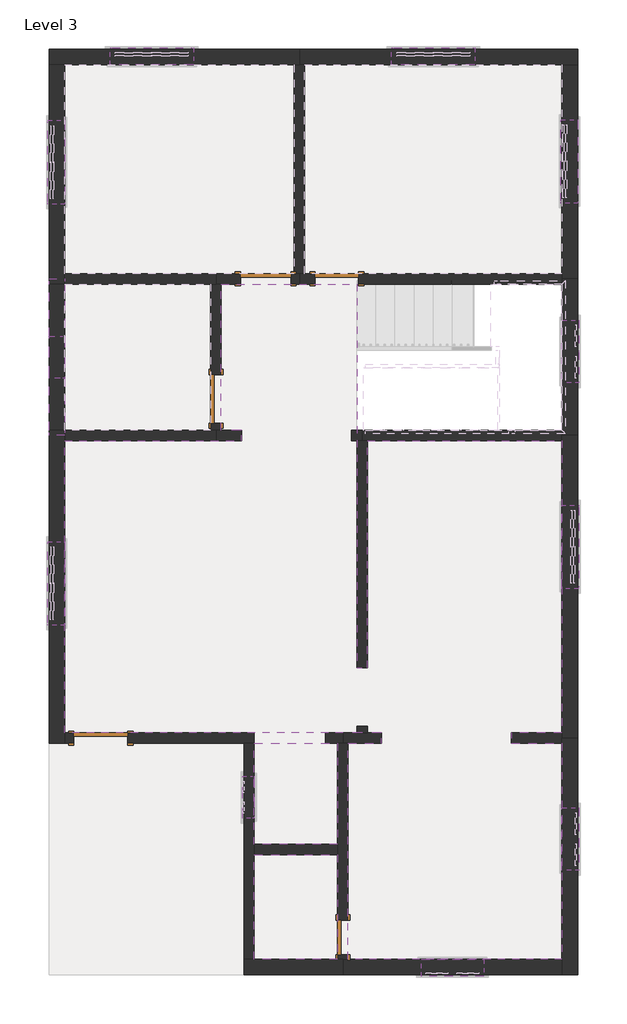
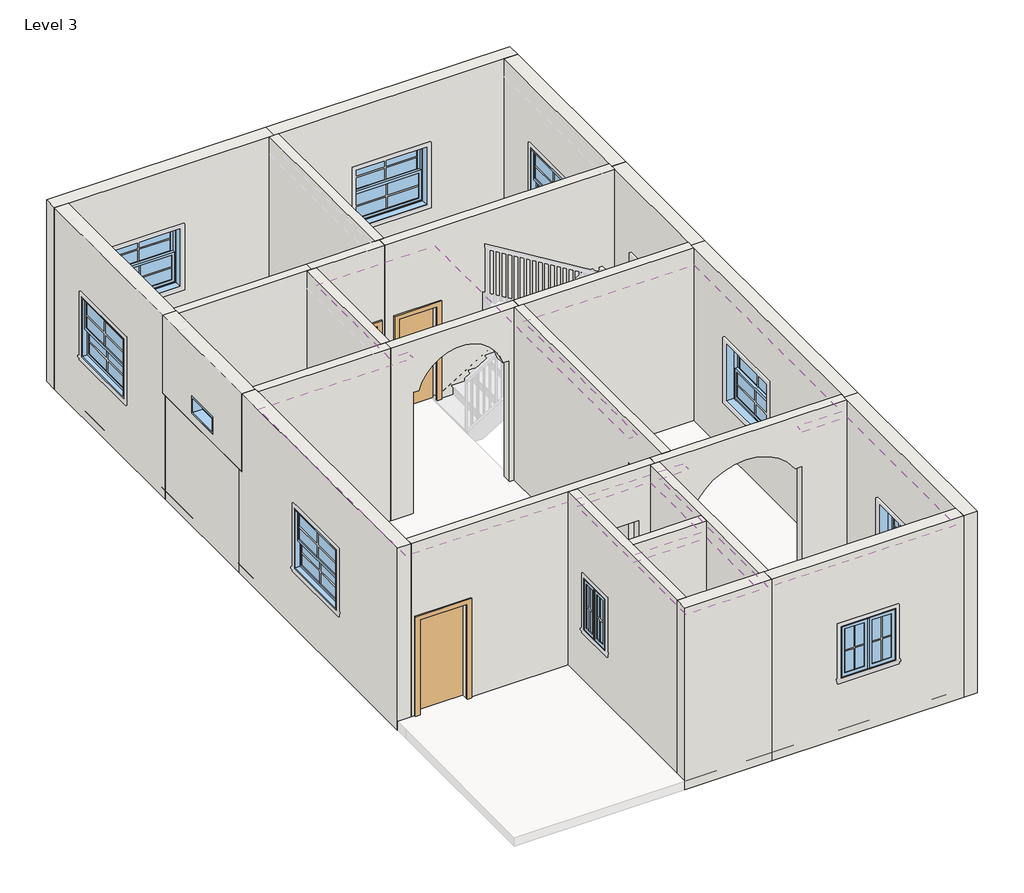
# One storey, part 1 of 2: 26 walls, 11 windows, 5 doors, 3 coverings.
"""IFC4 building model written with IfcOpenShell, lengths in millimetres."""

from ifc_helpers import new_model, si_unit, frame, origin, place, context, project, spatial, polyline, circle_curve, outline, extrude, faceted_brep, transform, mapped, element, save
from ifc_brep_helpers import plane_surface, revolved_surface, advanced_brep
from components import door_85c31a06, door_fe267433, door_77f51d0b, door_a6948854, door_ee35e093, fixed_2_8c8825d0, window_casement_double_2_fb285ced, window_casement_double_3_90de19e9, window_double_hung_4_eadb0177, window_double_hung_4_aab3aae7

model = new_model("IFC4")

# Units and contexts
model_context = context("Model", 3, world=origin())
ifc_project = project(units=[si_unit("LENGTHUNIT", "METRE", prefix="MILLI")], contexts=[model_context])

# Site, building, storey
site = spatial("IfcSite", under=ifc_project)
building = spatial("IfcBuilding", under=site)
storey = spatial("IfcBuildingStorey", under=building, Name="Level 3", Elevation=6400.8)

# Coverings
placement = place(None, origin())
element("IfcCovering", 1, ObjectType="2' x 4' ACT System", at=placement, inside=storey, context=model_context, shape_type="SweptSolid", body=[
    extrude(outline(polyline([(1592.635938, -3451.4142637), (1592.635938, -6601.0142637), (-1531.564062, -6601.0142637), (-1531.564062, -3451.4142637), (-1042.9877715, -3451.4142637), (-1042.9877715, -3299.0142637), (-1607.764062, -3299.0142637), (-5671.764062, -3299.0142637), (-5671.764062, 968.1857363), (-3538.164062, 968.1857363), (-3088.5741654, 968.1857363), (-3088.5741654, 1120.5857363), (-3385.764062, 1120.5857363), (-3385.764062, 3254.1857363), (-2242.764062, 3254.1857363), (-1404.564062, 3254.1857363), (-1404.564062, -2346.4297845), (-1252.164062, -2346.4297845), (-1252.164062, 968.1857363), (1592.635938, 968.1857363), (1592.635938, -3299.0142637), (852.655246, -3299.0142637), (852.655246, -3451.4142637), (1592.635938, -3451.4142637)])), frame((0.0, 0.0, 9448.8), z_axis=(0.0, 0.0, 1.0), x_axis=(1.0, 0.0, 0.0)), (0.0, 0.0, 1.0), 57.15),
])
element("IfcCovering", 2, ObjectType="2' x 4' ACT System", at=placement, inside=storey, context=model_context, shape_type="SweptSolid", body=[
    extrude(outline(polyline([(-2903.164062, -4924.6142637), (-2903.164062, -3451.4142637), (-1683.964062, -3451.4142637), (-1683.964062, -4924.6142637), (-2903.164062, -4924.6142637)])), frame((0.0, 0.0, 9448.8), z_axis=(0.0, 0.0, 1.0), x_axis=(1.0, 0.0, 0.0)), (0.0, 0.0, 1.0), 57.15),
])
element("IfcCovering", 3, ObjectType="2' x 4' ACT System", at=placement, inside=storey, context=model_context, shape_type="SweptSolid", body=[
    extrude(outline(polyline([(-2903.164062, -6601.0142637), (-2903.164062, -5077.0142637), (-1683.964062, -5077.0142637), (-1683.964062, -6601.0142637), (-2903.164062, -6601.0142637)])), frame((0.0, 0.0, 9448.8), z_axis=(0.0, 0.0, 1.0), x_axis=(1.0, 0.0, 0.0)), (0.0, 0.0, 1.0), 57.15),
])

# Doors
door_shape = door_85c31a06(model_context)
element("IfcDoor", 4, ObjectType="Single-Flush : 1'8\"", at=placement, inside=storey, context=model_context, shape_type="MappedRepresentation", body=[
    mapped(door_shape, transform((-1607.764062, -6283.5142637, 6553.2), x_axis=(0.0, -1.0, 0.0), y_axis=(1.0, 0.0, 0.0), z_axis=(0.0, 0.0, 1.0))),
])
door_2_shape = door_fe267433(model_context)
element("IfcDoor", 5, ObjectType="Single-Flush : 2'1\"", at=placement, inside=storey, context=model_context, shape_type="MappedRepresentation", body=[
    mapped(door_2_shape, transform((-1696.664062, 3330.3857363, 6553.2), x_axis=(-1.0, 0.0, 0.0), y_axis=(0.0, -1.0, 0.0), z_axis=(0.0, 0.0, 1.0))),
])
door_3_shape = door_77f51d0b(model_context)
element("IfcDoor", 6, ObjectType="Single-Flush : 2'4\"", at=placement, inside=storey, context=model_context, shape_type="MappedRepresentation", body=[
    mapped(door_3_shape, transform((-3461.964062, 1577.7857363, 6553.2), x_axis=(0.0, -1.0, 0.0), y_axis=(1.0, 0.0, 0.0), z_axis=(0.0, 0.0, 1.0))),
])
door_4_shape = door_a6948854(model_context)
element("IfcDoor", 7, ObjectType="Single-Flush : 2'5\"", at=placement, inside=storey, context=model_context, shape_type="MappedRepresentation", body=[
    mapped(door_4_shape, transform((-2738.064062, 3330.3857363, 6553.2), x_axis=(1.0, 0.0, 0.0), y_axis=(0.0, 1.0, 0.0), z_axis=(0.0, 0.0, 1.0))),
])
door_5_shape = door_ee35e093(model_context)
element("IfcDoor", 8, ObjectType="Single-Flush : 2'7\"", at=placement, inside=storey, context=model_context, shape_type="MappedRepresentation", body=[
    mapped(door_5_shape, transform((-5144.714062, -3375.2142637, 6553.2), x_axis=(-1.0, 0.0, 0.0), y_axis=(0.0, -1.0, 0.0), z_axis=(0.0, 0.0, 1.0))),
])

# Walls
element("IfcWall", 9, ObjectType="Generic - 6\"", at=placement, inside=storey, context=model_context, shape_type="Brep", body=[
    faceted_brep([(-2318.964062, 6454.5857363, 6553.2), (-2318.964062, 3406.5857363, 6553.2), (-2318.964062, 3406.5857363, 9753.6), (-2318.964062, 6454.5857363, 9753.6), (-2166.564062, 6454.5857363, 6553.2), (-2166.564062, 6454.5857363, 9753.6), (-2166.564062, 3406.5857363, 9753.6), (-2166.564062, 3406.5857363, 6553.2), (-2242.764062, 6454.5857363, 6553.2), (-2242.764062, 3406.5857363, 6553.2), (-2242.764062, 3406.5857363, 9753.6), (-2242.764062, 6454.5857363, 9753.6)], [[[0, 1, 2, 3]], [[4, 5, 6, 7]], [[1, 0, 8, 4, 7, 9]], [[3, 2, 10, 6, 5, 11]], [[0, 3, 11, 5, 4, 8]], [[2, 1, 9, 7, 6, 10]]]),
])
element("IfcWall", 10, ObjectType="Generic - 6\"", at=placement, inside=storey, context=model_context, shape_type="Brep", body=[
    faceted_brep([(-5671.764062, 3254.1857363, 9753.6), (-5671.764062, 3254.1857363, 8382.0), (-5671.764062, 3254.1857363, 6553.2), (-3538.164062, 3254.1857363, 6553.2), (-3461.964062, 3254.1857363, 6553.2), (-3461.964062, 3254.1857363, 9753.6), (-3538.164062, 3254.1857363, 9753.6), (-5671.764062, 3406.5857363, 6553.2), (-5671.764062, 3406.5857363, 9753.6), (-3461.964062, 3406.5857363, 9753.6), (-3461.964062, 3406.5857363, 6553.2), (-5671.764062, 3330.3857363, 9753.6)], [[[0, 1, 2, 3, 4, 5, 6]], [[7, 8, 9, 10]], [[4, 3, 2, 7, 10]], [[5, 4, 10, 9]], [[0, 6, 5, 9, 8, 11]], [[0, 11, 8, 7, 2, 1]]]),
])
element("IfcWall", 11, ObjectType="Generic - 6\"", at=placement, inside=storey, context=model_context, shape_type="Brep", body=[
    faceted_brep([(-5671.764062, 968.1857363, 9753.6), (-5671.764062, 968.1857363, 6553.2), (-3461.964062, 968.1857363, 6553.2), (-3461.964062, 968.1857363, 9753.6), (-5671.764062, 1120.5857363, 6553.2), (-5671.764062, 1120.5857363, 8382.0), (-5671.764062, 1120.5857363, 9753.6), (-3538.164062, 1120.5857363, 9753.6), (-3461.964062, 1120.5857363, 9753.6), (-3461.964062, 1120.5857363, 6553.2), (-3538.164062, 1120.5857363, 6553.2), (-5671.764062, 1044.3857363, 9753.6)], [[[0, 1, 2, 3]], [[4, 5, 6, 7, 8, 9, 10]], [[2, 1, 4, 10, 9]], [[3, 2, 9, 8]], [[0, 3, 8, 7, 6, 11]], [[0, 11, 6, 5, 4, 1]]]),
])
element("IfcWall", 12, ObjectType="Generic - 6\"", at=placement, inside=storey, context=model_context, shape_type="Brep", body=[
    faceted_brep([(-1404.564062, 968.1857363, 6553.2), (-1404.564062, -2346.4297845, 6553.2), (-1404.564062, -2346.4297845, 9017.0), (-1404.564062, -3197.4142637, 9017.0), (-1404.564062, -3197.4142637, 8839.2), (-1404.564062, -3197.4142637, 6553.2), (-1404.564062, -3299.0142637, 6553.2), (-1404.564062, -3299.0142637, 9753.6), (-1404.564062, 968.1857363, 9753.6), (-1252.164062, -2346.4297845, 6553.2), (-1252.164062, 968.1857363, 6553.2), (-1252.164062, 968.1857363, 9753.6), (-1252.164062, -3299.0142637, 9753.6), (-1252.164062, -3299.0142637, 6553.2), (-1252.164062, -3197.4142637, 6553.2), (-1252.164062, -3197.4142637, 8839.2), (-1252.164062, -3197.4142637, 9017.0), (-1252.164062, -2346.4297845, 9017.0), (-1328.364062, 968.1857363, 6553.2), (-1328.364062, 968.1857363, 9753.6)], [[[0, 1, 2, 3, 4, 5, 6, 7, 8]], [[9, 10, 11, 12, 13, 14, 15, 16, 17]], [[7, 6, 13, 12]], [[1, 0, 18, 10, 9]], [[8, 7, 12, 11, 19]], [[2, 1, 9, 17]], [[3, 2, 17, 16]], [[3, 16, 15, 14, 5, 4]], [[6, 5, 14, 13]], [[0, 8, 19, 11, 10, 18]]]),
])
element("IfcWall", 13, ObjectType="Generic - 6\"", at=placement, inside=storey, context=model_context, shape_type="Brep", body=[
    faceted_brep([(-2903.164062, -3451.4142637, 8839.2), (-1865.8319448, -3451.4142637, 8839.2), (-1865.8319448, -3451.4142637, 6553.2), (-1683.964062, -3451.4142637, 6553.2), (-1607.764062, -3451.4142637, 6553.2), (-1607.764062, -3451.4142637, 9753.6), (-1683.964062, -3451.4142637, 9753.6), (-2903.164062, -3451.4142637, 9753.6), (-3055.564062, -3451.4142637, 9753.6), (-5671.764062, -3451.4142637, 9753.6), (-5671.764062, -3451.4142637, 6553.2), (-5538.414062, -3451.4142637, 6553.2), (-5538.414062, -3451.4142637, 8382.0), (-4751.014062, -3451.4142637, 8382.0), (-4751.014062, -3451.4142637, 6553.2), (-3055.564062, -3451.4142637, 6553.2), (-2903.164062, -3451.4142637, 6553.2), (-1865.8319448, -3299.0142637, 8839.2), (-2903.164062, -3299.0142637, 8839.2), (-2903.164062, -3299.0142637, 6553.2), (-4751.014062, -3299.0142637, 6553.2), (-4751.014062, -3299.0142637, 8382.0), (-5538.414062, -3299.0142637, 8382.0), (-5538.414062, -3299.0142637, 6553.2), (-5671.764062, -3299.0142637, 6553.2), (-5671.764062, -3299.0142637, 9753.6), (-1607.764062, -3299.0142637, 9753.6), (-1607.764062, -3299.0142637, 6553.2), (-1865.8319448, -3299.0142637, 6553.2)], [[[0, 1, 2, 3, 4, 5, 6, 7, 8, 9, 10, 11, 12, 13, 14, 15, 16]], [[17, 18, 19, 20, 21, 22, 23, 24, 25, 26, 27, 28]], [[17, 1, 0, 18]], [[1, 17, 28, 2]], [[22, 12, 11, 23]], [[12, 22, 21, 13]], [[13, 21, 20, 14]], [[10, 24, 23, 11]], [[27, 4, 3, 2, 28]], [[19, 16, 15, 14, 20]], [[5, 4, 27, 26]], [[9, 8, 7, 6, 5, 26, 25]], [[10, 9, 25, 24]], [[18, 0, 16, 19]]]),
])
element("IfcWall", 14, ObjectType="Generic - 6\"", at=placement, inside=storey, context=model_context, shape_type="Brep", body=[
    faceted_brep([(-3055.564062, -3451.4142637, 6553.2), (-3055.564062, -6601.0142637, 6553.2), (-3055.564062, -6601.0142637, 9753.6), (-3055.564062, -3451.4142637, 9753.6), (-3055.564062, -3934.0142637, 8534.4), (-3055.564062, -4543.6142637, 8534.4), (-3055.564062, -4543.6142637, 7620.0), (-3055.564062, -3934.0142637, 7620.0), (-2903.164062, -3451.4142637, 6553.2), (-2903.164062, -3451.4142637, 8839.2), (-2903.164062, -3451.4142637, 9753.6), (-2903.164062, -4924.6142637, 9753.6), (-2903.164062, -5077.0142637, 9753.6), (-2903.164062, -6601.0142637, 9753.6), (-2903.164062, -6601.0142637, 6553.2), (-2903.164062, -5077.0142637, 6553.2), (-2903.164062, -4924.6142637, 6553.2), (-2903.164062, -3934.0142637, 8534.4), (-2903.164062, -3934.0142637, 7620.0), (-2903.164062, -4543.6142637, 7620.0), (-2903.164062, -4543.6142637, 8534.4)], [[[0, 1, 2, 3], [4, 5, 6, 7]], [[8, 9, 10, 11, 12, 13, 14, 15, 16], [17, 18, 19, 20]], [[1, 0, 8, 16, 15, 14]], [[3, 2, 13, 12, 11, 10]], [[2, 1, 14, 13]], [[18, 17, 4, 7]], [[19, 18, 7, 6]], [[20, 19, 6, 5]], [[17, 20, 5, 4]], [[0, 3, 10, 9, 8]]]),
])
element("IfcWall", 15, ObjectType="Generic - 6\"", at=placement, inside=storey, context=model_context, shape_type="Brep", body=[
    faceted_brep([(-1683.964062, -6601.0142637, 9753.6), (-1683.964062, -5077.0142637, 9753.6), (-1683.964062, -4924.6142637, 9753.6), (-1683.964062, -3451.4142637, 9753.6), (-1683.964062, -3451.4142637, 6553.2), (-1683.964062, -4924.6142637, 6553.2), (-1683.964062, -5077.0142637, 6553.2), (-1683.964062, -6029.5142637, 6553.2), (-1683.964062, -6029.5142637, 8382.0), (-1683.964062, -6537.5142637, 8382.0), (-1683.964062, -6537.5142637, 6553.2), (-1683.964062, -6601.0142637, 6553.2), (-1531.564062, -3451.4142637, 9753.6), (-1531.564062, -6601.0142637, 9753.6), (-1531.564062, -6601.0142637, 6553.2), (-1531.564062, -6537.5142637, 6553.2), (-1531.564062, -6537.5142637, 8382.0), (-1531.564062, -6029.5142637, 8382.0), (-1531.564062, -6029.5142637, 6553.2), (-1531.564062, -3451.4142637, 6553.2), (-1607.764062, -6601.0142637, 6553.2), (-1607.764062, -3451.4142637, 6553.2), (-1607.764062, -6601.0142637, 9753.6), (-1607.764062, -3451.4142637, 9753.6)], [[[0, 1, 2, 3, 4, 5, 6, 7, 8, 9, 10, 11]], [[12, 13, 14, 15, 16, 17, 18, 19]], [[14, 20, 11, 10, 15]], [[4, 21, 19, 18, 7, 6, 5]], [[3, 2, 1, 0, 22, 13, 12, 23]], [[9, 16, 15, 10]], [[16, 9, 8, 17]], [[17, 8, 7, 18]], [[0, 11, 20, 14, 13, 22]], [[4, 3, 23, 12, 19, 21]]]),
])
element("IfcWall", 16, ObjectType="Generic - 6\"", at=placement, inside=storey, context=model_context, shape_type="SweptSolid", body=[
    extrude(outline(polyline([(-1683.964062, -5077.0142637), (-2903.164062, -5077.0142637), (-2903.164062, -4924.6142637), (-1683.964062, -4924.6142637), (-1683.964062, -5077.0142637)])), frame((0.0, 0.0, 6553.2), z_axis=(0.0, 0.0, 1.0), x_axis=(1.0, 0.0, 0.0)), (0.0, 0.0, 1.0), 3200.4),
])
element("IfcWall", 17, ObjectType="Generic - 6\"", at=placement, inside=storey, context=model_context, shape_type="Brep", body=[
    faceted_brep([(-3538.164062, 1120.5857363, 9753.6), (-3538.164062, 3254.1857363, 9753.6), (-3538.164062, 3254.1857363, 6553.2), (-3538.164062, 1933.3857363, 6553.2), (-3538.164062, 1933.3857363, 8382.0), (-3538.164062, 1222.1857363, 8382.0), (-3538.164062, 1222.1857363, 6553.2), (-3538.164062, 1120.5857363, 6553.2), (-3385.764062, 3254.1857363, 9753.6), (-3385.764062, 1120.5857363, 9753.6), (-3385.764062, 1120.5857363, 6553.2), (-3385.764062, 1222.1857363, 6553.2), (-3385.764062, 1222.1857363, 8382.0), (-3385.764062, 1933.3857363, 8382.0), (-3385.764062, 1933.3857363, 6553.2), (-3385.764062, 3254.1857363, 6553.2), (-3461.964062, 3254.1857363, 6553.2), (-3461.964062, 1120.5857363, 6553.2), (-3461.964062, 1120.5857363, 9753.6), (-3461.964062, 3254.1857363, 9753.6)], [[[0, 1, 2, 3, 4, 5, 6, 7]], [[8, 9, 10, 11, 12, 13, 14, 15]], [[2, 16, 15, 14, 3]], [[10, 17, 7, 6, 11]], [[1, 0, 18, 9, 8, 19]], [[12, 5, 4, 13]], [[13, 4, 3, 14]], [[5, 12, 11, 6]], [[2, 1, 19, 8, 15, 16]], [[0, 7, 17, 10, 9, 18]]]),
])
element("IfcWall", 18, ObjectType="Generic - 6\"", at=placement, inside=storey, context=model_context, shape_type="Brep", body=[
    faceted_brep([(-2242.764062, 3254.1857363, 6553.2), (-2014.164062, 3254.1857363, 6553.2), (-2014.164062, 3254.1857363, 8382.0), (-1379.164062, 3254.1857363, 8382.0), (-1379.164062, 3254.1857363, 6553.2), (1592.635938, 3254.1857363, 6553.2), (1592.635938, 3254.1857363, 9753.6), (-2242.764062, 3254.1857363, 9753.6), (-2014.164062, 3406.5857363, 8382.0), (-2014.164062, 3406.5857363, 6553.2), (-2166.564062, 3406.5857363, 6553.2), (-2242.764062, 3406.5857363, 6553.2), (-2242.764062, 3406.5857363, 9753.6), (-2166.564062, 3406.5857363, 9753.6), (1592.635938, 3406.5857363, 9753.6), (1592.635938, 3406.5857363, 6553.2), (-1379.164062, 3406.5857363, 6553.2), (-1379.164062, 3406.5857363, 8382.0), (1592.635938, 3330.3857363, 6553.2), (1592.635938, 3330.3857363, 9753.6)], [[[0, 1, 2, 3, 4, 5, 6, 7]], [[8, 9, 10, 11, 12, 13, 14, 15, 16, 17]], [[16, 15, 18, 5, 4]], [[11, 10, 9, 1, 0]], [[7, 6, 19, 14, 13, 12]], [[0, 7, 12, 11]], [[6, 5, 18, 15, 14, 19]], [[4, 3, 17, 16]], [[3, 2, 8, 17]], [[2, 1, 9, 8]]]),
])
element("IfcWall", 19, ObjectType="Generic - 6\"", at=placement, inside=storey, context=model_context, shape_type="Brep", body=[
    faceted_brep([(1592.635938, 968.1857363, 9753.6), (-1252.164062, 968.1857363, 9753.6), (-1328.364062, 968.1857363, 9753.6), (-1328.364062, 968.1857363, 6553.2), (-1252.164062, 968.1857363, 6553.2), (1592.635938, 968.1857363, 6553.2), (1592.635938, 1120.5857363, 9753.6), (1592.635938, 1120.5857363, 6553.2), (-1328.364062, 1120.5857363, 6553.2), (-1328.364062, 1120.5857363, 9753.6), (1592.635938, 1044.3857363, 9753.6), (1592.635938, 1044.3857363, 6553.2)], [[[0, 1, 2, 3, 4, 5]], [[6, 7, 8, 9]], [[2, 1, 0, 10, 6, 9]], [[5, 4, 3, 8, 7, 11]], [[2, 9, 8, 3]], [[0, 5, 11, 7, 6, 10]]]),
])
element("IfcWall", 20, ObjectType="Generic - 6\"", at=placement, inside=storey, context=model_context, shape_type="AdvancedBrep", body=[
    advanced_brep(
    [(1592.635938, -3451.4142637, 9753.6), (-1531.564062, -3451.4142637, 9753.6), (-1607.764062, -3451.4142637, 9753.6), (-1607.764062, -3451.4142637, 6553.2), (-1531.564062, -3451.4142637, 6553.2), (-1042.9877715, -3451.4142637, 6553.2), (-1042.9877715, -3451.4142637, 8839.2), (-909.3649468, -3451.4142637, 8839.2), (732.5205767, -3451.4142637, 8839.2), (852.655246, -3451.4142637, 8839.2), (852.655246, -3451.4142637, 6553.2), (1592.635938, -3451.4142637, 6553.2), (-1607.764062, -3299.0142637, 9753.6), (-1404.564062, -3299.0142637, 9753.6), (-1252.164062, -3299.0142637, 9753.6), (1592.635938, -3299.0142637, 9753.6), (1592.635938, -3299.0142637, 6553.2), (852.655246, -3299.0142637, 6553.2), (852.655246, -3299.0142637, 8839.2), (732.5205767, -3299.0142637, 8839.2), (-909.3649468, -3299.0142637, 8839.2), (-1042.9877715, -3299.0142637, 8839.2), (-1042.9877715, -3299.0142637, 6553.2), (-1252.164062, -3299.0142637, 6553.2), (-1404.564062, -3299.0142637, 6553.2), (-1607.764062, -3299.0142637, 6553.2), (1592.635938, -3375.2142637, 9753.6), (1592.635938, -3375.2142637, 6553.2)],
    [
        (0, 1),
        (1, 2),
        (2, 3),
        (3, 4),
        (4, 5),
        (5, 6),
        (6, 7),
        (7, 8, circle_curve(frame((-88.4221851, -3451.4142637, 8303.4141821), z_axis=(0.0, 1.0, 0.0), x_axis=(-1.0, 0.0, 0.0)), 980.3129402)),
        (8, 9),
        (9, 10),
        (10, 11),
        (11, 0),
        (12, 13),
        (13, 14),
        (14, 15),
        (15, 16),
        (16, 17),
        (17, 18),
        (18, 19),
        (19, 20, circle_curve(frame((-88.4221851, -3299.0142637, 8303.4141821), z_axis=(0.0, -1.0, 0.0), x_axis=(-1.0, 0.0, 0.0)), 980.3129402)),
        (20, 21),
        (21, 22),
        (22, 23),
        (23, 24),
        (24, 25),
        (25, 12),
        (0, 26),
        (26, 15),
        (12, 2),
        (9, 18),
        (17, 10),
        (5, 22),
        (21, 6),
        (7, 20),
        (19, 8),
        (3, 25),
        (16, 27),
        (27, 11),
    ],
    [
        plane_surface(frame((1706.935938, -3451.4142637, 9753.6), z_axis=(0.0, -1.0, 0.0), x_axis=(-1.0, 0.0, 0.0))),
        plane_surface(frame((1706.935938, -3299.0142637, 9753.6), z_axis=(0.0, 1.0, 0.0), x_axis=(1.0, 0.0, 0.0))),
        plane_surface(frame((1706.935938, -3451.4142637, 9753.6), z_axis=(0.0, 0.0, 1.0), x_axis=(0.0, 1.0, 0.0))),
        plane_surface(frame((852.655246, -3451.4142637, 8577.980621), z_axis=(-1.0, 0.0, 0.0), x_axis=(0.0, 1.0, 0.0))),
        plane_surface(frame((-1042.9877715, -3451.4142637, 6888.7784957), z_axis=(1.0, 0.0, 0.0), x_axis=(0.0, 1.0, 0.0))),
        revolved_surface(polyline([(-1068.7351253, -3299.0142637, 8303.4141821), (-1068.7351253, -3451.4142637, 8303.4141821)]), (-88.4221851, -3299.0142637, 8303.4141821), (0.0, 1.0, 0.0)),
        plane_surface(frame((-1607.764062, -3451.4142637, 6553.2), z_axis=(0.0, 0.0, -1.0), x_axis=(0.0, 1.0, 0.0))),
        plane_surface(frame((456.9071606, -3451.4142637, 6553.2), z_axis=(0.0, 0.0, -1.0), x_axis=(0.0, 1.0, 0.0))),
        plane_surface(frame((-1607.764062, -3451.4142637, 9753.6), z_axis=(-1.0, 0.0, 0.0), x_axis=(0.0, 1.0, 0.0))),
        plane_surface(frame((1592.635938, 6454.5857363, 6553.2), z_axis=(1.0, 0.0, 0.0), x_axis=(0.0, -1.0, 0.0))),
        plane_surface(frame((-1042.9877715, -3299.0142637, 8839.2), z_axis=(0.0, 0.0, -1.0), x_axis=(-1.0, 0.0, 0.0))),
    ],
    [
        (0, [[1, 2, 3, 4, 5, 6, 7, 8, 9, 10, 11, 12]]),
        (1, [[13, 14, 15, 16, 17, 18, 19, 20, 21, 22, 23, 24, 25, 26]]),
        (2, [[-2, -1, 27, 28, -15, -14, -13, 29]]),
        (3, [[30, -18, 31, -10]]),
        (4, [[32, -22, 33, -6]]),
        (5, [[-8, 34, -20, 35]]),
        (6, [[36, -25, -24, -23, -32, -5, -4]]),
        (7, [[37, 38, -11, -31, -17]]),
        (8, [[-3, -29, -26, -36]]),
        (9, [[-12, -38, -37, -16, -28, -27]]),
        (10, [[-33, -21, -34, -7]]),
        (10, [[-30, -9, -35, -19]]),
    ],
),
])
element("IfcWall", 21, ObjectType="Generic - 6\"", at=placement, inside=storey, context=model_context, shape_type="Brep", body=[
    faceted_brep([(-2369.764062, 3254.1857363, 8382.0), (-2369.764062, 3254.1857363, 6553.2), (-2242.764062, 3254.1857363, 6553.2), (-2242.764062, 3254.1857363, 9753.6), (-3385.764062, 3254.1857363, 9753.6), (-3461.964062, 3254.1857363, 9753.6), (-3461.964062, 3254.1857363, 6553.2), (-3385.764062, 3254.1857363, 6553.2), (-3106.364062, 3254.1857363, 6553.2), (-3106.364062, 3254.1857363, 8382.0), (-2242.764062, 3406.5857363, 6553.2), (-2318.964062, 3406.5857363, 6553.2), (-2369.764062, 3406.5857363, 6553.2), (-2369.764062, 3406.5857363, 8382.0), (-3106.364062, 3406.5857363, 8382.0), (-3106.364062, 3406.5857363, 6553.2), (-3461.964062, 3406.5857363, 6553.2), (-3461.964062, 3406.5857363, 9753.6), (-2318.964062, 3406.5857363, 9753.6), (-2242.764062, 3406.5857363, 9753.6)], [[[0, 1, 2, 3, 4, 5, 6, 7, 8, 9]], [[10, 11, 12, 13, 14, 15, 16, 17, 18, 19]], [[2, 1, 12, 11, 10]], [[8, 7, 6, 16, 15]], [[3, 2, 10, 19]], [[5, 4, 3, 19, 18, 17]], [[6, 5, 17, 16]], [[15, 14, 9, 8]], [[14, 13, 0, 9]], [[13, 12, 1, 0]]]),
])
element("IfcWall", 22, ObjectType="Generic - 6\"", at=placement, inside=storey, context=model_context, shape_type="AdvancedBrep", body=[
    advanced_brep(
    [(-1328.364062, 968.1857363, 9753.6), (-1404.564062, 968.1857363, 9753.6), (-3461.964062, 968.1857363, 9753.6), (-3461.964062, 968.1857363, 6553.2), (-3088.5741654, 968.1857363, 6553.2), (-3088.5741654, 968.1857363, 8839.2), (-2990.069581, 968.1857363, 8839.2), (-1595.0493956, 968.1857363, 8839.2), (-1480.764062, 968.1857363, 8839.2), (-1480.764062, 968.1857363, 6553.2), (-1404.564062, 968.1857363, 6553.2), (-1328.364062, 968.1857363, 6553.2), (-3461.964062, 1120.5857363, 9753.6), (-3385.764062, 1120.5857363, 9753.6), (-1328.364062, 1120.5857363, 9753.6), (-1328.364062, 1120.5857363, 6553.2), (-1480.764062, 1120.5857363, 6553.2), (-1480.764062, 1120.5857363, 8839.2), (-1595.0493956, 1120.5857363, 8839.2), (-2990.069581, 1120.5857363, 8839.2), (-3088.5741654, 1120.5857363, 8839.2), (-3088.5741654, 1120.5857363, 6553.2), (-3385.764062, 1120.5857363, 6553.2), (-3461.964062, 1120.5857363, 6553.2)],
    [
        (0, 1),
        (1, 2),
        (2, 3),
        (3, 4),
        (4, 5),
        (5, 6),
        (6, 7, circle_curve(frame((-2292.5594883, 968.1857363, 8661.4), z_axis=(0.0, 1.0, 0.0), x_axis=(-1.0, 0.0, 0.0)), 719.8146771)),
        (7, 8),
        (8, 9),
        (9, 10),
        (10, 11),
        (11, 0),
        (12, 13),
        (13, 14),
        (14, 15),
        (15, 16),
        (16, 17),
        (17, 18),
        (18, 19, circle_curve(frame((-2292.5594883, 1120.5857363, 8661.4), z_axis=(0.0, -1.0, 0.0), x_axis=(-1.0, 0.0, 0.0)), 719.8146771)),
        (19, 20),
        (20, 21),
        (21, 22),
        (22, 23),
        (23, 12),
        (6, 19),
        (18, 7),
        (15, 11),
        (9, 16),
        (0, 14),
        (12, 2),
        (3, 23),
        (21, 4),
        (5, 20),
        (17, 8),
    ],
    [
        plane_surface(frame((-3012.3741654, 968.1857363, 8661.4), z_axis=(0.0, -1.0, 0.0), x_axis=(0.0, 0.0, 1.0))),
        plane_surface(frame((-3012.3741654, 1120.5857363, 8661.4), z_axis=(0.0, 1.0, 0.0), x_axis=(0.0, 0.0, -1.0))),
        revolved_surface(polyline([(-3012.3741654, 1120.5857363, 8661.4), (-3012.3741654, 968.1857363, 8661.4)]), (-2292.5594883, 1120.5857363, 8661.4), (0.0, 1.0, 0.0)),
        plane_surface(frame((-1572.7448112, 968.1857363, 6553.2), z_axis=(0.0, 0.0, -1.0), x_axis=(0.0, 1.0, 0.0))),
        plane_surface(frame((-1328.364062, 968.1857363, 9753.6), z_axis=(0.0, 0.0, 1.0), x_axis=(0.0, 1.0, 0.0))),
        plane_surface(frame((-3461.964062, 968.1857363, 6553.2), z_axis=(0.0, 0.0, -1.0), x_axis=(0.0, 1.0, 0.0))),
        plane_surface(frame((-1328.364062, 968.1857363, 6553.2), z_axis=(1.0, 0.0, 0.0), x_axis=(0.0, 1.0, 0.0))),
        plane_surface(frame((-3461.964062, 968.1857363, 9753.6), z_axis=(-1.0, 0.0, 0.0), x_axis=(0.0, 1.0, 0.0))),
        plane_surface(frame((-3088.5741654, 1120.5857363, 8839.2), z_axis=(0.0, 0.0, -1.0), x_axis=(-1.0, 0.0, 0.0))),
        plane_surface(frame((-3088.5741654, 1120.5857363, 8839.2), z_axis=(1.0, 0.0, 0.0), x_axis=(0.0, 0.0, -1.0))),
        plane_surface(frame((-1480.764062, 968.1857363, 8839.2), z_axis=(-1.0, 0.0, 0.0), x_axis=(0.0, 0.0, -1.0))),
    ],
    [
        (0, [[1, 2, 3, 4, 5, 6, 7, 8, 9, 10, 11, 12]]),
        (1, [[13, 14, 15, 16, 17, 18, 19, 20, 21, 22, 23, 24]]),
        (2, [[-7, 25, -19, 26]]),
        (3, [[27, -11, -10, 28, -16]]),
        (4, [[-2, -1, 29, -14, -13, 30]]),
        (5, [[31, -23, -22, 32, -4]]),
        (6, [[-12, -27, -15, -29]]),
        (7, [[-3, -30, -24, -31]]),
        (8, [[33, -20, -25, -6]]),
        (8, [[34, -8, -26, -18]]),
        (9, [[-33, -5, -32, -21]]),
        (10, [[-34, -17, -28, -9]]),
    ],
),
])
element("IfcWall", 23, ObjectType="Generic - 9\"", at=placement, inside=storey, context=model_context, shape_type="Brep", body=[
    faceted_brep([(-5900.364062, 6454.5857363, 6553.2), (-5671.764062, 6454.5857363, 6553.2), (-2318.964062, 6454.5857363, 6553.2), (-2242.764062, 6454.5857363, 6553.2), (-2242.764062, 6454.5857363, 9753.6), (-2318.964062, 6454.5857363, 9753.6), (-5671.764062, 6454.5857363, 9753.6), (-5900.364062, 6454.5857363, 9753.6), (-3792.164062, 6454.5857363, 8686.8), (-3792.164062, 6454.5857363, 7620.0), (-5011.364062, 6454.5857363, 7620.0), (-5011.364062, 6454.5857363, 8686.8), (-5900.364062, 6683.1857363, 6553.2), (-5900.364062, 6683.1857363, 9753.6), (-2242.764062, 6683.1857363, 9753.6), (-2242.764062, 6683.1857363, 6553.2), (-3792.164062, 6683.1857363, 8686.8), (-5011.364062, 6683.1857363, 8686.8), (-5011.364062, 6683.1857363, 7620.0), (-3792.164062, 6683.1857363, 7620.0)], [[[0, 1, 2, 3, 4, 5, 6, 7], [8, 9, 10, 11]], [[12, 13, 14, 15], [16, 17, 18, 19]], [[3, 2, 1, 0, 12, 15]], [[4, 3, 15, 14]], [[7, 6, 5, 4, 14, 13]], [[0, 7, 13, 12]], [[9, 8, 16, 19]], [[10, 9, 19, 18]], [[11, 10, 18, 17]], [[8, 11, 17, 16]]]),
])
element("IfcWall", 24, ObjectType="Generic - 9\"", at=placement, inside=storey, context=model_context, shape_type="Brep", body=[
    faceted_brep([(1592.635938, 6454.5857363, 6553.2), (1592.635938, 3406.5857363, 6553.2), (1592.635938, 3330.3857363, 6553.2), (1592.635938, 3330.3857363, 9753.6), (1592.635938, 3406.5857363, 9753.6), (1592.635938, 6454.5857363, 9753.6), (1592.635938, 5654.4857363, 8686.8), (1592.635938, 4435.2857363, 8686.8), (1592.635938, 4435.2857363, 7620.0), (1592.635938, 5654.4857363, 7620.0), (1821.235938, 6454.5857363, 6553.2), (1821.235938, 6454.5857363, 9753.6), (1821.235938, 3330.3857363, 9753.6), (1821.235938, 3330.3857363, 6553.2), (1821.235938, 5654.4857363, 8686.8), (1821.235938, 5654.4857363, 7620.0), (1821.235938, 4435.2857363, 7620.0), (1821.235938, 4435.2857363, 8686.8)], [[[0, 1, 2, 3, 4, 5], [6, 7, 8, 9]], [[10, 11, 12, 13], [14, 15, 16, 17]], [[2, 1, 0, 10, 13]], [[3, 2, 13, 12]], [[5, 4, 3, 12, 11]], [[0, 5, 11, 10]], [[15, 14, 6, 9]], [[16, 15, 9, 8]], [[17, 16, 8, 7]], [[14, 17, 7, 6]]]),
])
element("IfcWall", 25, ObjectType="Generic - 9\"", at=placement, inside=storey, context=model_context, shape_type="Brep", body=[
    faceted_brep([(1592.635938, -6601.0142637, 6553.2), (-1531.564062, -6601.0142637, 6553.2), (-1607.764062, -6601.0142637, 6553.2), (-1607.764062, -6601.0142637, 9753.6), (-1531.564062, -6601.0142637, 9753.6), (1592.635938, -6601.0142637, 9753.6), (-464.764062, -6601.0142637, 8534.4), (-464.764062, -6601.0142637, 7620.0), (449.635938, -6601.0142637, 7620.0), (449.635938, -6601.0142637, 8534.4), (1592.635938, -6829.6142637, 6553.2), (1592.635938, -6829.6142637, 9753.6), (-1607.764062, -6829.6142637, 9753.6), (-1607.764062, -6829.6142637, 6553.2), (-464.764062, -6829.6142637, 8534.4), (449.635938, -6829.6142637, 8534.4), (449.635938, -6829.6142637, 7620.0), (-464.764062, -6829.6142637, 7620.0)], [[[0, 1, 2, 3, 4, 5], [6, 7, 8, 9]], [[10, 11, 12, 13], [14, 15, 16, 17]], [[2, 1, 0, 10, 13]], [[3, 2, 13, 12]], [[5, 4, 3, 12, 11]], [[0, 5, 11, 10]], [[7, 6, 14, 17]], [[8, 7, 17, 16]], [[9, 8, 16, 15]], [[6, 9, 15, 14]]]),
])
element("IfcWall", 26, ObjectType="Generic - 9\"", at=placement, inside=storey, context=model_context, shape_type="Brep", body=[
    faceted_brep([(-5900.364062, 6454.5857363, 6553.2), (-5900.364062, 3254.1857363, 6553.2), (-5900.364062, 3254.1857363, 8382.0), (-5900.364062, 3330.3857363, 8382.0), (-5900.364062, 3330.3857363, 9753.6), (-5900.364062, 6454.5857363, 9753.6), (-5900.364062, 4422.5857363, 8686.8), (-5900.364062, 4422.5857363, 7620.0), (-5900.364062, 5641.7857363, 7620.0), (-5900.364062, 5641.7857363, 8686.8), (-5671.764062, 6454.5857363, 6553.2), (-5671.764062, 6454.5857363, 9753.6), (-5671.764062, 3406.5857363, 9753.6), (-5671.764062, 3330.3857363, 9753.6), (-5671.764062, 3330.3857363, 8382.0), (-5671.764062, 3254.1857363, 8382.0), (-5671.764062, 3254.1857363, 6553.2), (-5671.764062, 3406.5857363, 6553.2), (-5671.764062, 4422.5857363, 8686.8), (-5671.764062, 5641.7857363, 8686.8), (-5671.764062, 5641.7857363, 7620.0), (-5671.764062, 4422.5857363, 7620.0)], [[[0, 1, 2, 3, 4, 5], [6, 7, 8, 9]], [[10, 11, 12, 13, 14, 15, 16, 17], [18, 19, 20, 21]], [[1, 0, 10, 17, 16]], [[5, 4, 13, 12, 11]], [[0, 5, 11, 10]], [[7, 6, 18, 21]], [[8, 7, 21, 20]], [[9, 8, 20, 19]], [[6, 9, 19, 18]], [[4, 3, 14, 13]], [[14, 3, 2, 15]], [[2, 1, 16, 15]]]),
])
element("IfcWall", 27, ObjectType="Generic - 9\"", at=placement, inside=storey, context=model_context, shape_type="Brep", body=[
    faceted_brep([(-2242.764062, 6454.5857363, 6553.2), (-2166.564062, 6454.5857363, 6553.2), (1592.635938, 6454.5857363, 6553.2), (1821.235938, 6454.5857363, 6553.2), (1821.235938, 6454.5857363, 9753.6), (1592.635938, 6454.5857363, 9753.6), (-2166.564062, 6454.5857363, 9753.6), (-2242.764062, 6454.5857363, 9753.6), (322.635938, 6454.5857363, 8686.8), (322.635938, 6454.5857363, 7620.0), (-896.564062, 6454.5857363, 7620.0), (-896.564062, 6454.5857363, 8686.8), (-2242.764062, 6683.1857363, 6553.2), (-2242.764062, 6683.1857363, 9753.6), (1821.235938, 6683.1857363, 9753.6), (1821.235938, 6683.1857363, 6553.2), (322.635938, 6683.1857363, 8686.8), (-896.564062, 6683.1857363, 8686.8), (-896.564062, 6683.1857363, 7620.0), (322.635938, 6683.1857363, 7620.0)], [[[0, 1, 2, 3, 4, 5, 6, 7], [8, 9, 10, 11]], [[12, 13, 14, 15], [16, 17, 18, 19]], [[3, 2, 1, 0, 12, 15]], [[7, 6, 5, 4, 14, 13]], [[0, 7, 13, 12]], [[4, 3, 15, 14]], [[8, 11, 17, 16]], [[11, 10, 18, 17]], [[10, 9, 19, 18]], [[9, 8, 16, 19]]]),
])
element("IfcWall", 28, ObjectType="Generic - 9\"", at=placement, inside=storey, context=model_context, shape_type="Brep", body=[
    faceted_brep([(-1607.764062, -6601.0142637, 6553.2), (-1683.964062, -6601.0142637, 6553.2), (-2903.164062, -6601.0142637, 6553.2), (-3055.564062, -6601.0142637, 6553.2), (-3055.564062, -6601.0142637, 9753.6), (-2903.164062, -6601.0142637, 9753.6), (-1683.964062, -6601.0142637, 9753.6), (-1607.764062, -6601.0142637, 9753.6), (-1607.764062, -6829.6142637, 6553.2), (-1607.764062, -6829.6142637, 9753.6), (-3055.564062, -6829.6142637, 9753.6), (-3055.564062, -6829.6142637, 6553.2)], [[[0, 1, 2, 3, 4, 5, 6, 7]], [[8, 9, 10, 11]], [[3, 2, 1, 0, 8, 11]], [[7, 6, 5, 4, 10, 9]], [[0, 7, 9, 8]], [[4, 3, 11, 10]]]),
])
element("IfcWall", 29, ObjectType="Generic - 9\"", at=placement, inside=storey, context=model_context, shape_type="Brep", body=[
    faceted_brep([(1592.635938, 3330.3857363, 6553.2), (1592.635938, 3254.1857363, 6553.2), (1592.635938, 1120.5857363, 6553.2), (1592.635938, 1044.3857363, 6553.2), (1592.635938, 1044.3857363, 9753.6), (1592.635938, 1120.5857363, 9753.6), (1592.635938, 3254.1857363, 9753.6), (1592.635938, 3330.3857363, 9753.6), (1592.635938, 1812.7357363, 8534.4), (1592.635938, 1812.7357363, 7620.0), (1592.635938, 2727.1357363, 7620.0), (1592.635938, 2727.1357363, 8534.4), (1821.235938, 3330.3857363, 6553.2), (1821.235938, 3330.3857363, 9753.6), (1821.235938, 1044.3857363, 9753.6), (1821.235938, 1044.3857363, 6553.2), (1821.235938, 1812.7357363, 8534.4), (1821.235938, 2727.1357363, 8534.4), (1821.235938, 2727.1357363, 7620.0), (1821.235938, 1812.7357363, 7620.0)], [[[0, 1, 2, 3, 4, 5, 6, 7], [8, 9, 10, 11]], [[12, 13, 14, 15], [16, 17, 18, 19]], [[3, 2, 1, 0, 12, 15]], [[4, 3, 15, 14]], [[7, 6, 5, 4, 14, 13]], [[0, 7, 13, 12]], [[8, 11, 17, 16]], [[11, 10, 18, 17]], [[10, 9, 19, 18]], [[9, 8, 16, 19]]]),
])
element("IfcWall", 30, ObjectType="Generic - 9\"", at=placement, inside=storey, context=model_context, shape_type="Brep", body=[
    faceted_brep([(1592.635938, 1044.3857363, 6553.2), (1592.635938, 968.1857363, 6553.2), (1592.635938, -3299.0142637, 6553.2), (1592.635938, -3375.2142637, 6553.2), (1592.635938, -3375.2142637, 9753.6), (1592.635938, -3299.0142637, 9753.6), (1592.635938, 968.1857363, 9753.6), (1592.635938, 1044.3857363, 9753.6), (1592.635938, 28.3857363, 8686.8), (1592.635938, -1190.8142637, 8686.8), (1592.635938, -1190.8142637, 7620.0), (1592.635938, 28.3857363, 7620.0), (1821.235938, 1044.3857363, 6553.2), (1821.235938, 1044.3857363, 9753.6), (1821.235938, -3375.2142637, 9753.6), (1821.235938, -3375.2142637, 6553.2), (1821.235938, 28.3857363, 8686.8), (1821.235938, 28.3857363, 7620.0), (1821.235938, -1190.8142637, 7620.0), (1821.235938, -1190.8142637, 8686.8)], [[[0, 1, 2, 3, 4, 5, 6, 7], [8, 9, 10, 11]], [[12, 13, 14, 15], [16, 17, 18, 19]], [[3, 2, 1, 0, 12, 15]], [[4, 3, 15, 14]], [[7, 6, 5, 4, 14, 13]], [[0, 7, 13, 12]], [[16, 19, 9, 8]], [[19, 18, 10, 9]], [[18, 17, 11, 10]], [[17, 16, 8, 11]]]),
])
element("IfcWall", 31, ObjectType="Generic - 9\"", at=placement, inside=storey, context=model_context, shape_type="Brep", body=[
    faceted_brep([(1592.635938, -3375.2142637, 6553.2), (1592.635938, -3451.4142637, 6553.2), (1592.635938, -6601.0142637, 6553.2), (1592.635938, -6829.6142637, 6553.2), (1592.635938, -6829.6142637, 9753.6), (1592.635938, -6601.0142637, 9753.6), (1592.635938, -3451.4142637, 9753.6), (1592.635938, -3375.2142637, 9753.6), (1592.635938, -5305.6142637, 8534.4), (1592.635938, -5305.6142637, 7620.0), (1592.635938, -4391.2142637, 7620.0), (1592.635938, -4391.2142637, 8534.4), (1821.235938, -3375.2142637, 6553.2), (1821.235938, -3375.2142637, 9753.6), (1821.235938, -6829.6142637, 9753.6), (1821.235938, -6829.6142637, 6553.2), (1821.235938, -5305.6142637, 8534.4), (1821.235938, -4391.2142637, 8534.4), (1821.235938, -4391.2142637, 7620.0), (1821.235938, -5305.6142637, 7620.0)], [[[0, 1, 2, 3, 4, 5, 6, 7], [8, 9, 10, 11]], [[12, 13, 14, 15], [16, 17, 18, 19]], [[3, 2, 1, 0, 12, 15]], [[7, 6, 5, 4, 14, 13]], [[0, 7, 13, 12]], [[4, 3, 15, 14]], [[8, 11, 17, 16]], [[11, 10, 18, 17]], [[10, 9, 19, 18]], [[9, 8, 16, 19]]]),
])
element("IfcWall", 32, ObjectType="Generic - 9\"", at=placement, inside=storey, context=model_context, shape_type="Brep", body=[
    faceted_brep([(-5900.364062, 1120.5857363, 6553.2), (-5900.364062, -3451.4142637, 6553.2), (-5900.364062, -3451.4142637, 9753.6), (-5900.364062, 1044.3857363, 9753.6), (-5900.364062, 1044.3857363, 8382.0), (-5900.364062, 1120.5857363, 8382.0), (-5900.364062, -1724.2142637, 8686.8), (-5900.364062, -1724.2142637, 7620.0), (-5900.364062, -505.0142637, 7620.0), (-5900.364062, -505.0142637, 8686.8), (-5671.764062, 1120.5857363, 6553.2), (-5671.764062, 1120.5857363, 8382.0), (-5671.764062, 1044.3857363, 8382.0), (-5671.764062, 1044.3857363, 9753.6), (-5671.764062, 968.1857363, 9753.6), (-5671.764062, -3299.0142637, 9753.6), (-5671.764062, -3451.4142637, 9753.6), (-5671.764062, -3451.4142637, 6553.2), (-5671.764062, -3299.0142637, 6553.2), (-5671.764062, 968.1857363, 6553.2), (-5671.764062, -1724.2142637, 8686.8), (-5671.764062, -505.0142637, 8686.8), (-5671.764062, -505.0142637, 7620.0), (-5671.764062, -1724.2142637, 7620.0)], [[[0, 1, 2, 3, 4, 5], [6, 7, 8, 9]], [[10, 11, 12, 13, 14, 15, 16, 17, 18, 19], [20, 21, 22, 23]], [[1, 0, 10, 19, 18, 17]], [[3, 2, 16, 15, 14, 13]], [[2, 1, 17, 16]], [[6, 9, 21, 20]], [[9, 8, 22, 21]], [[8, 7, 23, 22]], [[7, 6, 20, 23]], [[4, 3, 13, 12]], [[4, 12, 11, 5]], [[0, 5, 11, 10]]]),
])
element("IfcWall", 33, ObjectType="Generic - 9\"", at=placement, inside=storey, context=model_context, shape_type="Brep", body=[
    faceted_brep([(-5900.364062, 3330.3857363, 8382.0), (-5900.364062, 3254.1857363, 8382.0), (-5900.364062, 1120.5857363, 8382.0), (-5900.364062, 1044.3857363, 8382.0), (-5900.364062, 1044.3857363, 9753.6), (-5900.364062, 3330.3857363, 9753.6), (-5900.364062, 1882.5857363, 8839.2), (-5900.364062, 1882.5857363, 8534.4), (-5900.364062, 2492.1857363, 8534.4), (-5900.364062, 2492.1857363, 8839.2), (-5671.764062, 3330.3857363, 8382.0), (-5671.764062, 3330.3857363, 9753.6), (-5671.764062, 3254.1857363, 9753.6), (-5671.764062, 1120.5857363, 9753.6), (-5671.764062, 1044.3857363, 9753.6), (-5671.764062, 1044.3857363, 8382.0), (-5671.764062, 1120.5857363, 8382.0), (-5671.764062, 3254.1857363, 8382.0), (-5671.764062, 1882.5857363, 8839.2), (-5671.764062, 2492.1857363, 8839.2), (-5671.764062, 2492.1857363, 8534.4), (-5671.764062, 1882.5857363, 8534.4)], [[[0, 1, 2, 3, 4, 5], [6, 7, 8, 9]], [[10, 11, 12, 13, 14, 15, 16, 17], [18, 19, 20, 21]], [[3, 2, 1, 0, 10, 17, 16, 15]], [[4, 3, 15, 14]], [[5, 4, 14, 13, 12, 11]], [[0, 5, 11, 10]], [[6, 9, 19, 18]], [[9, 8, 20, 19]], [[8, 7, 21, 20]], [[7, 6, 18, 21]]]),
])
element("IfcWall", 34, ObjectType="Generic - 9\"", at=placement, inside=storey, context=model_context, shape_type="SweptSolid", body=[
    extrude(outline(polyline([(-5900.364062, 1120.5857363), (-5900.364062, 3254.1857363), (-5671.764062, 3254.1857363), (-5671.764062, 1120.5857363), (-5900.364062, 1120.5857363)])), frame((0.0, 0.0, 6553.2), z_axis=(0.0, 0.0, 1.0), x_axis=(1.0, 0.0, 0.0)), (0.0, 0.0, 1.0), 1828.8),
])

# Windows
fixed_2_shape = fixed_2_8c8825d0(model_context)
element("IfcWindow", 35, ObjectType="Fixed : 2'", at=placement, inside=storey, context=model_context, shape_type="MappedRepresentation", body=[
    mapped(fixed_2_shape, transform((-5786.064062, 2149.2857363, 7620.0), x_axis=(0.0, -1.0, 0.0), y_axis=(1.0, 0.0, 0.0), z_axis=(0.0, 0.0, 1.0))),
])
window_casement_double_2_shape = window_casement_double_2_fb285ced(model_context)
element("IfcWindow", 36, ObjectType="Window-Casement-Double : 2'", at=placement, inside=storey, context=model_context, shape_type="MappedRepresentation", body=[
    mapped(window_casement_double_2_shape, transform((-2979.364062, -4238.8142637, 6705.6), x_axis=(0.0, 1.0, 0.0), y_axis=(-1.0, 0.0, 0.0), z_axis=(0.0, 0.0, 1.0))),
])
window_casement_double_3_shape = window_casement_double_3_90de19e9(model_context)
element("IfcWindow", 37, ObjectType="Window-Casement-Double : 3'", at=placement, inside=storey, context=model_context, shape_type="MappedRepresentation", body=[
    mapped(window_casement_double_3_shape, transform((1706.935938, -4848.4142637, 6705.6), x_axis=(0.0, -1.0, 0.0), y_axis=(1.0, 0.0, 0.0), z_axis=(0.0, 0.0, 1.0))),
])
element("IfcWindow", 38, ObjectType="Window-Casement-Double : 3'", at=placement, inside=storey, context=model_context, shape_type="MappedRepresentation", body=[
    mapped(window_casement_double_3_shape, transform((-7.564062, -6715.3142637, 6705.6), x_axis=(-1.0, 0.0, 0.0), y_axis=(0.0, -1.0, 0.0), z_axis=(0.0, 0.0, 1.0))),
])
element("IfcWindow", 39, ObjectType="Window-Casement-Double : 3'", at=placement, inside=storey, context=model_context, shape_type="MappedRepresentation", body=[
    mapped(window_casement_double_3_shape, transform((1706.935938, 2269.9357363, 6705.6), x_axis=(0.0, -1.0, 0.0), y_axis=(1.0, 0.0, 0.0), z_axis=(0.0, 0.0, 1.0))),
])
window_double_hung_4_shape = window_double_hung_4_eadb0177(model_context)
element("IfcWindow", 40, ObjectType="Window-Double-Hung : 4'", at=placement, inside=storey, context=model_context, shape_type="MappedRepresentation", body=[
    mapped(window_double_hung_4_shape, transform((-5786.064062, 5032.1857363, 6705.6), x_axis=(0.0, 1.0, 0.0), y_axis=(-1.0, 0.0, 0.0), z_axis=(0.0, 0.0, 1.0))),
])
element("IfcWindow", 41, ObjectType="Window-Double-Hung : 4'", at=placement, inside=storey, context=model_context, shape_type="MappedRepresentation", body=[
    mapped(window_double_hung_4_shape, transform((1706.935938, -581.2142637, 6705.6), x_axis=(0.0, -1.0, 0.0), y_axis=(1.0, 0.0, 0.0), z_axis=(0.0, 0.0, 1.0))),
])
element("IfcWindow", 42, ObjectType="Window-Double-Hung : 4'", at=placement, inside=storey, context=model_context, shape_type="MappedRepresentation", body=[
    mapped(window_double_hung_4_shape, transform((-5786.064062, -1114.6142637, 6705.6), x_axis=(0.0, 1.0, 0.0), y_axis=(-1.0, 0.0, 0.0), z_axis=(0.0, 0.0, 1.0))),
])
window_double_hung_4_2_shape = window_double_hung_4_aab3aae7(model_context)
element("IfcWindow", 43, ObjectType="Window-Double-Hung : 4'", at=placement, inside=storey, context=model_context, shape_type="MappedRepresentation", body=[
    mapped(window_double_hung_4_2_shape, transform((-4401.764062, 6568.8857363, 6705.6), x_axis=(-1.0, 0.0, 0.0), y_axis=(0.0, -1.0, 0.0), z_axis=(0.0, 0.0, 1.0))),
])
element("IfcWindow", 44, ObjectType="Window-Double-Hung : 4'", at=placement, inside=storey, context=model_context, shape_type="MappedRepresentation", body=[
    mapped(window_double_hung_4_2_shape, transform((-286.964062, 6568.8857363, 6705.6), x_axis=(-1.0, 0.0, 0.0), y_axis=(0.0, -1.0, 0.0), z_axis=(0.0, 0.0, 1.0))),
])
element("IfcWindow", 45, ObjectType="Window-Double-Hung : 4'", at=placement, inside=storey, context=model_context, shape_type="MappedRepresentation", body=[
    mapped(window_double_hung_4_2_shape, transform((1706.935938, 5044.8857363, 6705.6), x_axis=(0.0, -1.0, 0.0), y_axis=(1.0, 0.0, 0.0), z_axis=(0.0, 0.0, 1.0))),
])

save(model, "model.ifc")

# Revit data of these elements
# Type "2' x 4' ACT System"
#   Assembly Code = "C3030210"
#   built-in parameter 1002203 = 1 (stored number, unit not read)
#   built-in parameter 1002202 = 1 (stored number, unit not read)
#   Layers, outside or top first: 0' - 1 5/8" "Default" (function 1); 0' - 0 5/8" "Acoustic Ceiling Tile 24 x 48" (function 5)
# Type "Single-Flush : 1'8\""
#   Type Mark = "11"
#   Construction Type Id = "MDOOR"
#   Assembly Code = "C1020"
#   Analytic Construction = "Metal"
#   Thickness = 0' - 2"
#   Heat Transfer Coefficient (U) = 0.651978 BTU/(h·ft²·°F)
#   Height = 6' - 0"
#   Trim Projection Ext = 0' - 1"
#   Trim Projection Int = 0' - 1"
#   Trim Width = 0' - 3"
#   Width = 1' - 8"
#   Define Thermal Properties by = 1
#   Door Material = Door - Panel
#   Frame Material = Door - Frame
#   Visual Light Transmittance = 0
#   Solar Heat Gain Coefficient = 0
#   Function = (empty or 0)
#   Wall Closure = (empty or 0)
# Type "Single-Flush : 2'1\""
#   Type Mark = "9"
#   Construction Type Id = "MDOOR"
#   Assembly Code = "C1020"
#   Analytic Construction = "Metal"
#   Thickness = 0' - 2"
#   Heat Transfer Coefficient (U) = 0.651978 BTU/(h·ft²·°F)
#   Height = 6' - 0"
#   Trim Projection Ext = 0' - 1"
#   Trim Projection Int = 0' - 1"
#   Trim Width = 0' - 3"
#   Width = 2' - 1"
#   Define Thermal Properties by = 1
#   Door Material = Door - Panel
#   Frame Material = Door - Frame
#   Visual Light Transmittance = 0
#   Solar Heat Gain Coefficient = 0
#   Function = (empty or 0)
#   Wall Closure = (empty or 0)
# Type "Single-Flush : 2'4\""
#   Type Mark = "10"
#   Construction Type Id = "MDOOR"
#   Assembly Code = "C1020"
#   Analytic Construction = "Metal"
#   Thickness = 0' - 2"
#   Heat Transfer Coefficient (U) = 0.651978 BTU/(h·ft²·°F)
#   Height = 6' - 0"
#   Trim Projection Ext = 0' - 1"
#   Trim Projection Int = 0' - 1"
#   Trim Width = 0' - 3"
#   Width = 2' - 4"
#   Define Thermal Properties by = 1
#   Door Material = Door - Panel
#   Frame Material = Door - Frame
#   Visual Light Transmittance = 0
#   Solar Heat Gain Coefficient = 0
#   Function = (empty or 0)
#   Wall Closure = (empty or 0)
# Type "Single-Flush : 2'5\""
#   Type Mark = "8"
#   Construction Type Id = "MDOOR"
#   Assembly Code = "C1020"
#   Analytic Construction = "Metal"
#   Thickness = 0' - 2"
#   Heat Transfer Coefficient (U) = 0.651978 BTU/(h·ft²·°F)
#   Height = 6' - 0"
#   Trim Projection Ext = 0' - 1"
#   Trim Projection Int = 0' - 1"
#   Trim Width = 0' - 3"
#   Width = 2' - 5"
#   Define Thermal Properties by = 1
#   Door Material = Door - Panel
#   Frame Material = Door - Frame
#   Visual Light Transmittance = 0
#   Solar Heat Gain Coefficient = 0
#   Function = (empty or 0)
#   Wall Closure = (empty or 0)
# Type "Single-Flush : 2'7\""
#   Type Mark = "12"
#   Construction Type Id = "MDOOR"
#   Assembly Code = "C1020"
#   Analytic Construction = "Metal"
#   Thickness = 0' - 2"
#   Heat Transfer Coefficient (U) = 0.651978 BTU/(h·ft²·°F)
#   Height = 6' - 0"
#   Trim Projection Ext = 0' - 1"
#   Trim Projection Int = 0' - 1"
#   Trim Width = 0' - 3"
#   Width = 2' - 7"
#   Define Thermal Properties by = 1
#   Door Material = Door - Panel
#   Frame Material = Door - Frame
#   Visual Light Transmittance = 0
#   Solar Heat Gain Coefficient = 0
#   Function = (empty or 0)
#   Wall Closure = (empty or 0)
# Type "Generic - 6\""
#   Assembly Code = "B2010"
#   Layers, outside or top first: 0' - 6" no material (function 1)
# Type "Generic - 9\""
#   Assembly Code = "B2010"
#   Layers, outside or top first: 0' - 9" no material (function 1)
# Type "Fixed : 2'"
#   Type Mark = "21"
#   Construction Type Id = "GSP4R"
#   Assembly Code = "B2020100"
#   Analytic Construction = "1/8 in Pilkington single glazing"
#   Rough Height = 1' - 0"
#   Visual Light Transmittance = 0.9
#   Solar Heat Gain Coefficient = 0.78
#   Heat Transfer Coefficient (U) = 0.6496 BTU/(h·ft²·°F)
#   Height = 1' - 0"
#   Default Sill Height = 3' - 0"
#   Width = 2' - 0"
#   Window Inset = 0' - 0 3/4"
#   Define Thermal Properties by = 1
#   Glass Pane Material = Glass
#   Sash Material = Sash
#   Wall Closure = (empty or 0)
# Type "Window-Casement-Double : 2'"
#   Type Mark = "20"
#   Fire Rating = "0.5h"
#   Assembly Code = "B2020100"
#   Analytic Construction = "Double glazing - domestic"
#   Frame Extension [instance default] = 0' - 0 1/4"
#   Window Inset [instance default] = 0' - 0"
#   Wall Thickness [instance default] = 0' - 6"
#   Interior Wall Closure [instance default] = 0' - 2 1/4"
#   Half Width = 1' - 0"
#   Visual Light Transmittance = 0.81
#   Thermal Resistance (R) = 1.8146 (h·ft²·°F)/BTU
#   Solar Heat Gain Coefficient = 0.76
#   Rough Width = 2' - 0 1/2"
#   Rough Height = 3' - 0 1/2"
#   Height = 3' - 0"
#   Heat Transfer Coefficient (U) = 0.5511 BTU/(h·ft²·°F)
#   Exterior Wall Closure [instance default] = 0' - 1 1/4"
#   Extension Jamb [instance default] = 0' - 2 1/4"
#   Default Sill Height = 3' - 0"
#   Width = 2' - 0"
#   Muntin Visibility = yes
#   Interior Trim Visibility [instance default] = yes
#   Exterior Trim Visibility [instance default] = yes
#   Extension Jamb Visibility [instance default] = yes
#   Interior Trim Material = Wood - Stained
#   Muntin Pattern = Muntin Pattern_2x2 : Muntin Pattern_2x2
#   Interior Trim = Trim-Window-Interior-Flat : Picture Frame
#   Interior Frame Material = Wood - Stained
#   Glass Panel Material = Glass
#   Exterior Trim Material = Clad - White
#   Exterior Trim = Trim-Window-Exterior-Flat : with Sill
#   Exterior Frame Material = Clad - White
#   Wall Closure = (empty or 0)
# Type "Window-Casement-Double : 3'"
#   Type Mark = "19"
#   Fire Rating = "0.5h"
#   Assembly Code = "B2020100"
#   Analytic Construction = "Double glazing - domestic"
#   Frame Extension [instance default] = 0' - 0 1/4"
#   Window Inset [instance default] = 0' - 0"
#   Wall Thickness [instance default] = 0' - 6"
#   Interior Wall Closure [instance default] = 0' - 2 1/4"
#   Half Width = 1' - 6"
#   Visual Light Transmittance = 0.81
#   Thermal Resistance (R) = 1.8146 (h·ft²·°F)/BTU
#   Solar Heat Gain Coefficient = 0.76
#   Rough Width = 3' - 0 1/2"
#   Rough Height = 3' - 0 1/2"
#   Height = 3' - 0"
#   Heat Transfer Coefficient (U) = 0.5511 BTU/(h·ft²·°F)
#   Exterior Wall Closure [instance default] = 0' - 1 1/4"
#   Extension Jamb [instance default] = 0' - 2 1/4"
#   Default Sill Height = 3' - 0"
#   Width = 3' - 0"
#   Muntin Visibility = yes
#   Interior Trim Visibility [instance default] = yes
#   Exterior Trim Visibility [instance default] = yes
#   Extension Jamb Visibility [instance default] = yes
#   Interior Trim Material = Wood - Stained
#   Muntin Pattern = Muntin Pattern_2x2 : Muntin Pattern_2x2
#   Interior Trim = Trim-Window-Interior-Flat : Picture Frame
#   Interior Frame Material = Wood - Stained
#   Glass Panel Material = Glass
#   Exterior Trim Material = Clad - White
#   Exterior Trim = Trim-Window-Exterior-Flat : with Sill
#   Exterior Frame Material = Clad - White
#   Wall Closure = (empty or 0)
# Type "Window-Double-Hung : 4'"
#   Type Mark = "18"
#   Fire Rating = "0.5h"
#   Construction Type Id = "DG-DR"
#   Assembly Code = "B2020100"
#   Analytic Construction = "Double glazing - domestic"
#   Wall Thickness [instance default] = 0' - 6"
#   Window Inset [instance default] = 0' - 0"
#   Visual Light Transmittance = 0.81
#   Thermal Resistance (R) = 1.8146 (h·ft²·°F)/BTU
#   Solar Heat Gain Coefficient = 0.76
#   Muntin Width = 3' - 6"
#   Muntin Height = 1' - 5 1/8"
#   Interior Wall Closure [instance default] = 0' - 1 1/2"
#   Rough Width = 4' - 0 1/2"
#   Rough Height = 3' - 6 1/2"
#   Frame Extension [instance default] = 0' - 1 1/4"
#   Exterior Wall Closure [instance default] = 0' - 0 1/2"
#   Extension Jamb [instance default] = 0' - 1 1/2"
#   Heat Transfer Coefficient (U) = 0.5511 BTU/(h·ft²·°F)
#   Height = 3' - 6"
#   Width = 4' - 0"
#   Top Muntin Visibility = yes
#   Indicator Visibility [instance default] = yes
#   Extension Jamb Visibility [instance default] = yes
#   Interior Trim Visibility [instance default] = yes
#   Exterior Trim Visibility [instance default] = yes
#   Define Thermal Properties by = 1
#   Bottom Muntin Visibility = yes
#   Muntin Pattern = Muntin Pattern_2x2 : Muntin Pattern_2x2
#   Interior Trim Material = Wood - Stained
#   Interior Trim = Trim-Window-Interior-Flat : Picture Frame
#   Exterior Trim Material = Clad - White
#   Exterior Trim = Trim-Window-Exterior-Flat : with Sill
#   Glass Panel Material = Glass
#   Exterior Frame Material = Clad - White
#   Interior Frame Material = Wood - Stained
#   Wall Closure = (empty or 0)
# Elements 1, 2, 3 (IfcCovering, "2' x 4' ACT System")
#   Height Offset From Level = 10' - 0"
#   Phase Created = New Construction
#   Materials on its faces: "Acoustic Ceiling Tile 24 x 48", "Default"
# Element 4 (IfcDoor, "Single-Flush : 1'8\"")
#   Phase Created = New Construction
#   Materials on its faces: "Door - Frame", "Door - Panel"
# Element 5 (IfcDoor, "Single-Flush : 2'1\"")
#   Phase Created = New Construction
#   Materials on its faces: "Door - Frame", "Door - Panel"
# Element 6 (IfcDoor, "Single-Flush : 2'4\"")
#   Phase Created = New Construction
#   Materials on its faces: "Door - Frame", "Door - Panel"
# Element 7 (IfcDoor, "Single-Flush : 2'5\"")
#   Phase Created = New Construction
#   Materials on its faces: "Door - Frame", "Door - Panel"
# Element 8 (IfcDoor, "Single-Flush : 2'7\"")
#   Phase Created = New Construction
#   Materials on its faces: "Door - Frame", "Door - Panel"
# Elements 9, 17 (IfcWall, "Generic - 6\"")
#   built-in parameter 1001111 = 0' - 6"
#   Top Offset = 0' - 0"
#   Base Offset = 0' - 6"
#   Unconnected Height = 10' - 6"
#   wall height = 10' - 6"
#   Phase Created = New Construction
#   Base Constraint = Level 3
#   Materials on its faces: "Default Wall", "LAVENDER WHITE"
# Elements 10, 11, 14, 16, 22 (IfcWall, "Generic - 6\"")
#   built-in parameter 1001111 = 0' - 6"
#   Top Offset = 0' - 0"
#   Base Offset = 0' - 6"
#   Unconnected Height = 10' - 6"
#   wall height = 10' - 6"
#   Phase Created = New Construction
#   Base Constraint = Level 3
#   Materials on its faces: "Default Wall"
# Element 12 (IfcWall, "Generic - 6\"")
#   built-in parameter 1001111 = 0' - 6"
#   Top Offset = 0' - 0"
#   Base Offset = 0' - 6"
#   Unconnected Height = 10' - 6"
#   wall height = 10' - 6"
#   Phase Created = New Construction
#   Base Constraint = Level 3
#   Materials on its faces: "Default Wall", "LIVING ROOM WALL", "BURGUNDY COLOUR"
# Element 13 (IfcWall, "Generic - 6\"")
#   built-in parameter 1001111 = 0' - 6"
#   Top Offset = 0' - 0"
#   Base Offset = 0' - 6"
#   Unconnected Height = 10' - 6"
#   wall height = 10' - 6"
#   Phase Created = New Construction
#   Base Constraint = Level 3
#   Materials on its faces: "Default Wall", "DINING ROOM WALL", "BURGUNDY COLOUR"
